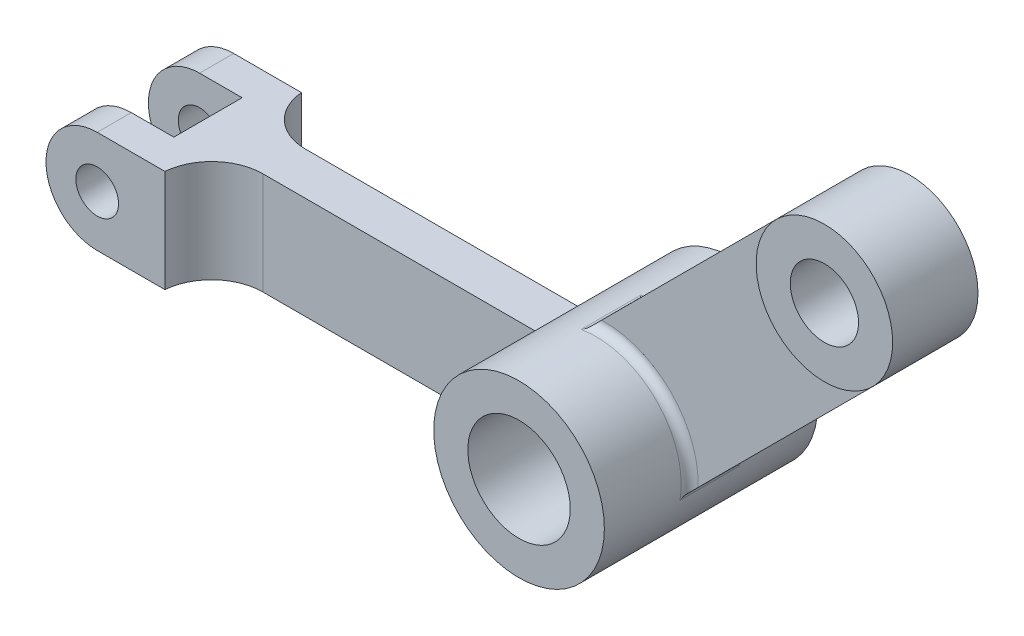
ISO-10303-21;
HEADER;
FILE_DESCRIPTION(('STEP AP214'),'2;1');
FILE_NAME('part.step','',(''),(''),'','','');
FILE_SCHEMA(('AUTOMOTIVE_DESIGN { 1 0 10303 214 1 1 1 1 }'));
ENDSEC;
DATA;
#1=APPLICATION_CONTEXT('core data for automotive mechanical design processes');
#2=APPLICATION_PROTOCOL_DEFINITION('international standard','automotive_design',2000,#1);
#3=PRODUCT_CONTEXT('',#1,'mechanical');
#4=PRODUCT('Part','Part','',(#3));
#5=PRODUCT_RELATED_PRODUCT_CATEGORY('part','',(#4));
#6=PRODUCT_DEFINITION_FORMATION('','',#4);
#7=PRODUCT_DEFINITION_CONTEXT('part definition',#1,'design');
#8=PRODUCT_DEFINITION('design','',#6,#7);
#9=PRODUCT_DEFINITION_SHAPE('','',#8);
#10=(LENGTH_UNIT() NAMED_UNIT(*) SI_UNIT(.MILLI.,.METRE.));
#11=(NAMED_UNIT(*) PLANE_ANGLE_UNIT() SI_UNIT($,.RADIAN.));
#12=(NAMED_UNIT(*) SI_UNIT($,.STERADIAN.) SOLID_ANGLE_UNIT());
#13=UNCERTAINTY_MEASURE_WITH_UNIT(LENGTH_MEASURE(1.E-05),#10,'distance_accuracy_value','');
#14=(GEOMETRIC_REPRESENTATION_CONTEXT(3) GLOBAL_UNCERTAINTY_ASSIGNED_CONTEXT((#13)) GLOBAL_UNIT_ASSIGNED_CONTEXT((#10,
#11,#12)) REPRESENTATION_CONTEXT('',''));
#15=CARTESIAN_POINT('',(0.,0.,0.));
#16=DIRECTION('',(0.,0.,1.));
#17=DIRECTION('',(1.,0.,0.));
#18=AXIS2_PLACEMENT_3D('',#15,#16,#17);
#19=CARTESIAN_POINT('',(0.,0.,25.));
#20=DIRECTION('',(0.,0.,1.));
#21=DIRECTION('',(1.,0.,0.));
#22=AXIS2_PLACEMENT_3D('',#19,#20,#21);
#23=PLANE('',#22);
#24=CARTESIAN_POINT('',(0.,0.,25.));
#25=DIRECTION('',(0.,0.,1.));
#26=DIRECTION('',(1.,0.,0.));
#27=AXIS2_PLACEMENT_3D('',#24,#25,#26);
#28=CIRCLE('',#27,10.);
#29=CARTESIAN_POINT('',(10.,0.,25.));
#30=VERTEX_POINT('',#29);
#31=EDGE_CURVE('E304',#30,#30,#28,.T.);
#32=ORIENTED_EDGE('',*,*,#31,.T.);
#33=EDGE_LOOP('',(#32));
#34=FACE_BOUND('',#33,.T.);
#35=CARTESIAN_POINT('',(0.,0.,25.));
#36=DIRECTION('',(0.,0.,1.));
#37=DIRECTION('',(1.,0.,0.));
#38=AXIS2_PLACEMENT_3D('',#35,#36,#37);
#39=CIRCLE('',#38,6.);
#40=CARTESIAN_POINT('',(6.,0.,25.));
#41=VERTEX_POINT('',#40);
#42=EDGE_CURVE('E299',#41,#41,#39,.T.);
#43=ORIENTED_EDGE('',*,*,#42,.F.);
#44=EDGE_LOOP('',(#43));
#45=FACE_BOUND('',#44,.T.);
#46=ADVANCED_FACE('F39',(#34,#45),#23,.T.);
#47=CARTESIAN_POINT('',(0.,0.,0.));
#48=DIRECTION('',(0.,0.,1.));
#49=DIRECTION('',(1.,0.,0.));
#50=AXIS2_PLACEMENT_3D('',#47,#48,#49);
#51=PLANE('',#50);
#52=CARTESIAN_POINT('',(0.,0.,0.));
#53=DIRECTION('',(0.,0.,1.));
#54=DIRECTION('',(1.,0.,0.));
#55=AXIS2_PLACEMENT_3D('',#52,#53,#54);
#56=CIRCLE('',#55,10.);
#57=CARTESIAN_POINT('',(10.,0.,0.));
#58=VERTEX_POINT('',#57);
#59=EDGE_CURVE('E305',#58,#58,#56,.T.);
#60=ORIENTED_EDGE('',*,*,#59,.F.);
#61=EDGE_LOOP('',(#60));
#62=FACE_BOUND('',#61,.T.);
#63=CARTESIAN_POINT('',(0.,0.,0.));
#64=DIRECTION('',(0.,0.,1.));
#65=DIRECTION('',(1.,0.,0.));
#66=AXIS2_PLACEMENT_3D('',#63,#64,#65);
#67=CIRCLE('',#66,6.);
#68=CARTESIAN_POINT('',(6.,0.,0.));
#69=VERTEX_POINT('',#68);
#70=EDGE_CURVE('E294',#69,#69,#67,.T.);
#71=ORIENTED_EDGE('',*,*,#70,.T.);
#72=EDGE_LOOP('',(#71));
#73=FACE_BOUND('',#72,.T.);
#74=ADVANCED_FACE('F412',(#62,#73),#51,.F.);
#75=CARTESIAN_POINT('',(0.,0.,25.));
#76=DIRECTION('',(0.,0.,-1.));
#77=DIRECTION('',(-1.,0.,0.));
#78=AXIS2_PLACEMENT_3D('',#75,#76,#77);
#79=CYLINDRICAL_SURFACE('',#78,10.);
#80=CARTESIAN_POINT('',(0.,0.,16.));
#81=DIRECTION('',(0.,0.,1.));
#82=DIRECTION('',(1.,0.,0.));
#83=AXIS2_PLACEMENT_3D('',#80,#81,#82);
#84=CIRCLE('',#83,10.);
#85=CARTESIAN_POINT('',(9.85099725970773,-1.71984097789032,16.));
#86=VERTEX_POINT('',#85);
#87=CARTESIAN_POINT('',(-1.71984097789032,9.85099725970773,16.));
#88=VERTEX_POINT('',#87);
#89=EDGE_CURVE('E339',#86,#88,#84,.T.);
#90=ORIENTED_EDGE('',*,*,#89,.T.);
#91=DIRECTION('',(0.,0.,-1.));
#92=VECTOR('',#91,1.);
#93=CARTESIAN_POINT('',(-1.71984097789032,9.85099725970773,25.));
#94=LINE('',#93,#92);
#95=CARTESIAN_POINT('',(-1.71984097789032,9.85099725970773,9.));
#96=VERTEX_POINT('',#95);
#97=EDGE_CURVE('E344',#88,#96,#94,.T.);
#98=ORIENTED_EDGE('',*,*,#97,.T.);
#99=CARTESIAN_POINT('',(0.,0.,9.));
#100=DIRECTION('',(0.,0.,1.));
#101=DIRECTION('',(1.,0.,0.));
#102=AXIS2_PLACEMENT_3D('',#99,#100,#101);
#103=CIRCLE('',#102,10.);
#104=CARTESIAN_POINT('',(9.85099725970773,-1.71984097789032,9.));
#105=VERTEX_POINT('',#104);
#106=EDGE_CURVE('E334',#96,#105,#103,.F.);
#107=ORIENTED_EDGE('',*,*,#106,.T.);
#108=DIRECTION('',(0.,0.,-1.));
#109=VECTOR('',#108,1.);
#110=CARTESIAN_POINT('',(9.85099725970773,-1.71984097789032,25.));
#111=LINE('',#110,#109);
#112=EDGE_CURVE('E340',#105,#86,#111,.F.);
#113=ORIENTED_EDGE('',*,*,#112,.T.);
#114=EDGE_LOOP('',(#90,#98,#107,#113));
#115=FACE_BOUND('',#114,.T.);
#116=DIRECTION('',(0.,0.,-1.));
#117=VECTOR('',#116,1.);
#118=CARTESIAN_POINT('',(-8.,6.,25.));
#119=LINE('',#118,#117);
#120=CARTESIAN_POINT('',(-8.,6.,15.));
#121=VERTEX_POINT('',#120);
#122=CARTESIAN_POINT('',(-8.,6.,10.));
#123=VERTEX_POINT('',#122);
#124=EDGE_CURVE('E312',#121,#123,#119,.T.);
#125=ORIENTED_EDGE('',*,*,#124,.F.);
#126=CARTESIAN_POINT('',(0.,0.,15.));
#127=DIRECTION('',(0.,0.,1.));
#128=DIRECTION('',(1.,0.,0.));
#129=AXIS2_PLACEMENT_3D('',#126,#127,#128);
#130=CIRCLE('',#129,10.);
#131=CARTESIAN_POINT('',(-8.,-6.,15.));
#132=VERTEX_POINT('',#131);
#133=EDGE_CURVE('E316',#121,#132,#130,.T.);
#134=ORIENTED_EDGE('',*,*,#133,.T.);
#135=DIRECTION('',(0.,0.,-1.));
#136=VECTOR('',#135,1.);
#137=CARTESIAN_POINT('',(-8.,-6.,25.));
#138=LINE('',#137,#136);
#139=CARTESIAN_POINT('',(-8.,-6.,10.));
#140=VERTEX_POINT('',#139);
#141=EDGE_CURVE('E317',#140,#132,#138,.F.);
#142=ORIENTED_EDGE('',*,*,#141,.F.);
#143=CARTESIAN_POINT('',(0.,0.,10.));
#144=DIRECTION('',(0.,0.,1.));
#145=DIRECTION('',(1.,0.,0.));
#146=AXIS2_PLACEMENT_3D('',#143,#144,#145);
#147=CIRCLE('',#146,10.);
#148=EDGE_CURVE('E308',#123,#140,#147,.T.);
#149=ORIENTED_EDGE('',*,*,#148,.F.);
#150=EDGE_LOOP('',(#125,#134,#142,#149));
#151=FACE_BOUND('',#150,.T.);
#152=ORIENTED_EDGE('',*,*,#31,.F.);
#153=EDGE_LOOP('',(#152));
#154=FACE_BOUND('',#153,.T.);
#155=ORIENTED_EDGE('',*,*,#59,.T.);
#156=EDGE_LOOP('',(#155));
#157=FACE_BOUND('',#156,.T.);
#158=ADVANCED_FACE('F414',(#115,#151,#154,#157),#79,.T.);
#159=CARTESIAN_POINT('',(0.,0.,25.));
#160=DIRECTION('',(0.,0.,-1.));
#161=DIRECTION('',(-1.,0.,0.));
#162=AXIS2_PLACEMENT_3D('',#159,#160,#161);
#163=CYLINDRICAL_SURFACE('',#162,6.);
#164=ORIENTED_EDGE('',*,*,#42,.T.);
#165=EDGE_LOOP('',(#164));
#166=FACE_BOUND('',#165,.T.);
#167=ORIENTED_EDGE('',*,*,#70,.F.);
#168=EDGE_LOOP('',(#167));
#169=FACE_BOUND('',#168,.T.);
#170=ADVANCED_FACE('F413',(#166,#169),#163,.F.);
#171=CARTESIAN_POINT('',(-46.,-6.,15.));
#172=DIRECTION('',(0.,1.,0.));
#173=DIRECTION('',(0.,0.,1.));
#174=AXIS2_PLACEMENT_3D('',#171,#172,#173);
#175=PLANE('',#174);
#176=DIRECTION('',(1.,0.,0.));
#177=VECTOR('',#176,1.);
#178=CARTESIAN_POINT('',(-46.,-6.,4.5));
#179=LINE('',#178,#177);
#180=CARTESIAN_POINT('',(-53.9333097995708,-6.,4.5));
#181=VERTEX_POINT('',#180);
#182=CARTESIAN_POINT('',(-46.,-6.,4.5));
#183=VERTEX_POINT('',#182);
#184=EDGE_CURVE('E267',#181,#183,#179,.T.);
#185=ORIENTED_EDGE('',*,*,#184,.T.);
#186=CARTESIAN_POINT('',(-40.0208696284493,-6.,4.));
#187=DIRECTION('',(0.,1.,0.));
#188=DIRECTION('',(0.,0.,1.));
#189=AXIS2_PLACEMENT_3D('',#186,#187,#188);
#190=CIRCLE('',#189,6.);
#191=CARTESIAN_POINT('',(-40.0208696284493,-6.,10.));
#192=VERTEX_POINT('',#191);
#193=EDGE_CURVE('E326',#183,#192,#190,.T.);
#194=ORIENTED_EDGE('',*,*,#193,.T.);
#195=DIRECTION('',(1.,0.,0.));
#196=VECTOR('',#195,1.);
#197=CARTESIAN_POINT('',(-46.,-6.,10.));
#198=LINE('',#197,#196);
#199=EDGE_CURVE('E283',#192,#140,#198,.T.);
#200=ORIENTED_EDGE('',*,*,#199,.T.);
#201=ORIENTED_EDGE('',*,*,#141,.T.);
#202=DIRECTION('',(1.,0.,0.));
#203=VECTOR('',#202,1.);
#204=CARTESIAN_POINT('',(-46.,-6.,15.));
#205=LINE('',#204,#203);
#206=CARTESIAN_POINT('',(-40.0208696284493,-6.,15.));
#207=VERTEX_POINT('',#206);
#208=EDGE_CURVE('E287',#207,#132,#205,.T.);
#209=ORIENTED_EDGE('',*,*,#208,.F.);
#210=CARTESIAN_POINT('',(-40.0208696284493,-6.,21.));
#211=DIRECTION('',(0.,1.,0.));
#212=DIRECTION('',(0.,0.,1.));
#213=AXIS2_PLACEMENT_3D('',#210,#211,#212);
#214=CIRCLE('',#213,6.);
#215=CARTESIAN_POINT('',(-46.,-6.,20.5));
#216=VERTEX_POINT('',#215);
#217=EDGE_CURVE('E333',#207,#216,#214,.T.);
#218=ORIENTED_EDGE('',*,*,#217,.T.);
#219=DIRECTION('',(1.,0.,0.));
#220=VECTOR('',#219,1.);
#221=CARTESIAN_POINT('',(-46.,-6.,20.5));
#222=LINE('',#221,#220);
#223=CARTESIAN_POINT('',(-53.9333097995708,-6.,20.5));
#224=VERTEX_POINT('',#223);
#225=EDGE_CURVE('E260',#224,#216,#222,.T.);
#226=ORIENTED_EDGE('',*,*,#225,.F.);
#227=DIRECTION('',(0.,0.,-1.));
#228=VECTOR('',#227,1.);
#229=CARTESIAN_POINT('',(-53.9333097995708,-6.,20.5));
#230=LINE('',#229,#228);
#231=CARTESIAN_POINT('',(-53.9333097995708,-6.,16.5));
#232=VERTEX_POINT('',#231);
#233=EDGE_CURVE('E284',#224,#232,#230,.T.);
#234=ORIENTED_EDGE('',*,*,#233,.T.);
#235=DIRECTION('',(1.,0.,0.));
#236=VECTOR('',#235,1.);
#237=CARTESIAN_POINT('',(-46.,-6.,16.5));
#238=LINE('',#237,#236);
#239=CARTESIAN_POINT('',(-48.9536388352292,-6.,16.5));
#240=VERTEX_POINT('',#239);
#241=EDGE_CURVE('E235',#232,#240,#238,.T.);
#242=ORIENTED_EDGE('',*,*,#241,.T.);
#243=DIRECTION('',(0.,0.,-1.));
#244=VECTOR('',#243,1.);
#245=CARTESIAN_POINT('',(-48.9536388352292,-6.,20.5));
#246=LINE('',#245,#244);
#247=CARTESIAN_POINT('',(-48.9536388352292,-6.,8.5));
#248=VERTEX_POINT('',#247);
#249=EDGE_CURVE('E244',#240,#248,#246,.T.);
#250=ORIENTED_EDGE('',*,*,#249,.T.);
#251=DIRECTION('',(-1.,0.,0.));
#252=VECTOR('',#251,1.);
#253=CARTESIAN_POINT('',(-46.,-6.,8.5));
#254=LINE('',#253,#252);
#255=CARTESIAN_POINT('',(-53.9333097995708,-6.,8.5));
#256=VERTEX_POINT('',#255);
#257=EDGE_CURVE('E237',#248,#256,#254,.T.);
#258=ORIENTED_EDGE('',*,*,#257,.T.);
#259=EDGE_CURVE('E277',#256,#181,#230,.T.);
#260=ORIENTED_EDGE('',*,*,#259,.T.);
#261=EDGE_LOOP('',(#185,#194,#200,#201,#209,#218,#226,#234,#242,#250,#258,#260));
#262=FACE_BOUND('',#261,.T.);
#263=ADVANCED_FACE('F424',(#262),#175,.F.);
#264=CARTESIAN_POINT('',(-46.,6.,15.));
#265=DIRECTION('',(0.,-1.,0.));
#266=DIRECTION('',(0.,0.,-1.));
#267=AXIS2_PLACEMENT_3D('',#264,#265,#266);
#268=PLANE('',#267);
#269=DIRECTION('',(-1.,0.,0.));
#270=VECTOR('',#269,1.);
#271=CARTESIAN_POINT('',(-46.,6.,15.));
#272=LINE('',#271,#270);
#273=CARTESIAN_POINT('',(-40.0208696284493,6.,15.));
#274=VERTEX_POINT('',#273);
#275=EDGE_CURVE('E293',#121,#274,#272,.T.);
#276=ORIENTED_EDGE('',*,*,#275,.F.);
#277=ORIENTED_EDGE('',*,*,#124,.T.);
#278=DIRECTION('',(-1.,0.,0.));
#279=VECTOR('',#278,1.);
#280=CARTESIAN_POINT('',(-46.,6.,10.));
#281=LINE('',#280,#279);
#282=CARTESIAN_POINT('',(-40.0208696284493,6.,10.));
#283=VERTEX_POINT('',#282);
#284=EDGE_CURVE('E292',#123,#283,#281,.T.);
#285=ORIENTED_EDGE('',*,*,#284,.T.);
#286=CARTESIAN_POINT('',(-40.0208696284493,6.,4.));
#287=DIRECTION('',(0.,-1.,0.));
#288=DIRECTION('',(0.,0.,-1.));
#289=AXIS2_PLACEMENT_3D('',#286,#287,#288);
#290=CIRCLE('',#289,6.);
#291=CARTESIAN_POINT('',(-46.,6.,4.5));
#292=VERTEX_POINT('',#291);
#293=EDGE_CURVE('E328',#283,#292,#290,.T.);
#294=ORIENTED_EDGE('',*,*,#293,.T.);
#295=DIRECTION('',(-1.,0.,0.));
#296=VECTOR('',#295,1.);
#297=CARTESIAN_POINT('',(-53.9333097995708,6.,4.5));
#298=LINE('',#297,#296);
#299=CARTESIAN_POINT('',(-53.9333097995708,6.,4.5));
#300=VERTEX_POINT('',#299);
#301=EDGE_CURVE('E258',#292,#300,#298,.T.);
#302=ORIENTED_EDGE('',*,*,#301,.T.);
#303=DIRECTION('',(0.,0.,-1.));
#304=VECTOR('',#303,1.);
#305=CARTESIAN_POINT('',(-53.9333097995708,6.,20.5));
#306=LINE('',#305,#304);
#307=CARTESIAN_POINT('',(-53.9333097995708,6.,8.5));
#308=VERTEX_POINT('',#307);
#309=EDGE_CURVE('E268',#308,#300,#306,.T.);
#310=ORIENTED_EDGE('',*,*,#309,.F.);
#311=DIRECTION('',(-1.,0.,0.));
#312=VECTOR('',#311,1.);
#313=CARTESIAN_POINT('',(-63.6938952559095,6.,8.5));
#314=LINE('',#313,#312);
#315=CARTESIAN_POINT('',(-48.9536388352292,6.,8.5));
#316=VERTEX_POINT('',#315);
#317=EDGE_CURVE('E191',#316,#308,#314,.T.);
#318=ORIENTED_EDGE('',*,*,#317,.F.);
#319=DIRECTION('',(0.,0.,-1.));
#320=VECTOR('',#319,1.);
#321=CARTESIAN_POINT('',(-48.9536388352292,6.,8.5));
#322=LINE('',#321,#320);
#323=CARTESIAN_POINT('',(-48.9536388352292,6.,16.5));
#324=VERTEX_POINT('',#323);
#325=EDGE_CURVE('E222',#324,#316,#322,.T.);
#326=ORIENTED_EDGE('',*,*,#325,.F.);
#327=DIRECTION('',(1.,0.,0.));
#328=VECTOR('',#327,1.);
#329=CARTESIAN_POINT('',(-48.9536388352292,6.,16.5));
#330=LINE('',#329,#328);
#331=CARTESIAN_POINT('',(-53.9333097995708,6.,16.5));
#332=VERTEX_POINT('',#331);
#333=EDGE_CURVE('E223',#332,#324,#330,.T.);
#334=ORIENTED_EDGE('',*,*,#333,.F.);
#335=CARTESIAN_POINT('',(-53.9333097995708,6.,20.5));
#336=VERTEX_POINT('',#335);
#337=EDGE_CURVE('E276',#336,#332,#306,.T.);
#338=ORIENTED_EDGE('',*,*,#337,.F.);
#339=DIRECTION('',(-1.,0.,0.));
#340=VECTOR('',#339,1.);
#341=CARTESIAN_POINT('',(-53.9333097995708,6.,20.5));
#342=LINE('',#341,#340);
#343=CARTESIAN_POINT('',(-46.,6.,20.5));
#344=VERTEX_POINT('',#343);
#345=EDGE_CURVE('E263',#344,#336,#342,.T.);
#346=ORIENTED_EDGE('',*,*,#345,.F.);
#347=CARTESIAN_POINT('',(-40.0208696284493,6.,21.));
#348=DIRECTION('',(0.,-1.,0.));
#349=DIRECTION('',(0.,0.,-1.));
#350=AXIS2_PLACEMENT_3D('',#347,#348,#349);
#351=CIRCLE('',#350,6.);
#352=EDGE_CURVE('E331',#344,#274,#351,.T.);
#353=ORIENTED_EDGE('',*,*,#352,.T.);
#354=EDGE_LOOP('',(#276,#277,#285,#294,#302,#310,#318,#326,#334,#338,#346,#353));
#355=FACE_BOUND('',#354,.T.);
#356=ADVANCED_FACE('F429',(#355),#268,.F.);
#357=CARTESIAN_POINT('',(0.,0.,15.));
#358=DIRECTION('',(0.,0.,1.));
#359=DIRECTION('',(1.,0.,0.));
#360=AXIS2_PLACEMENT_3D('',#357,#358,#359);
#361=PLANE('',#360);
#362=ORIENTED_EDGE('',*,*,#275,.T.);
#363=DIRECTION('',(0.,-1.,0.));
#364=VECTOR('',#363,1.);
#365=CARTESIAN_POINT('',(-40.0208696284493,-6.,15.));
#366=LINE('',#365,#364);
#367=EDGE_CURVE('E323',#274,#207,#366,.T.);
#368=ORIENTED_EDGE('',*,*,#367,.T.);
#369=ORIENTED_EDGE('',*,*,#208,.T.);
#370=ORIENTED_EDGE('',*,*,#133,.F.);
#371=EDGE_LOOP('',(#362,#368,#369,#370));
#372=FACE_BOUND('',#371,.T.);
#373=ADVANCED_FACE('F433',(#372),#361,.T.);
#374=CARTESIAN_POINT('',(0.,0.,10.));
#375=DIRECTION('',(0.,0.,1.));
#376=DIRECTION('',(1.,0.,0.));
#377=AXIS2_PLACEMENT_3D('',#374,#375,#376);
#378=PLANE('',#377);
#379=ORIENTED_EDGE('',*,*,#199,.F.);
#380=DIRECTION('',(0.,1.,0.));
#381=VECTOR('',#380,1.);
#382=CARTESIAN_POINT('',(-40.0208696284493,0.,10.));
#383=LINE('',#382,#381);
#384=EDGE_CURVE('E321',#192,#283,#383,.T.);
#385=ORIENTED_EDGE('',*,*,#384,.T.);
#386=ORIENTED_EDGE('',*,*,#284,.F.);
#387=ORIENTED_EDGE('',*,*,#148,.T.);
#388=EDGE_LOOP('',(#379,#385,#386,#387));
#389=FACE_BOUND('',#388,.T.);
#390=ADVANCED_FACE('F434',(#389),#378,.F.);
#391=CARTESIAN_POINT('',(-53.9333097995708,0.,20.5));
#392=DIRECTION('',(0.,0.,-1.));
#393=DIRECTION('',(-1.,0.,0.));
#394=AXIS2_PLACEMENT_3D('',#391,#392,#393);
#395=CYLINDRICAL_SURFACE('',#394,6.);
#396=ORIENTED_EDGE('',*,*,#259,.F.);
#397=CARTESIAN_POINT('',(-53.9333097995708,0.,8.5));
#398=DIRECTION('',(0.,0.,-1.));
#399=DIRECTION('',(-1.,0.,0.));
#400=AXIS2_PLACEMENT_3D('',#397,#398,#399);
#401=CIRCLE('',#400,6.);
#402=EDGE_CURVE('E245',#256,#308,#401,.T.);
#403=ORIENTED_EDGE('',*,*,#402,.T.);
#404=ORIENTED_EDGE('',*,*,#309,.T.);
#405=CARTESIAN_POINT('',(-53.9333097995708,0.,4.5));
#406=DIRECTION('',(0.,0.,1.));
#407=DIRECTION('',(1.,0.,0.));
#408=AXIS2_PLACEMENT_3D('',#405,#406,#407);
#409=CIRCLE('',#408,6.);
#410=EDGE_CURVE('E255',#300,#181,#409,.T.);
#411=ORIENTED_EDGE('',*,*,#410,.T.);
#412=EDGE_LOOP('',(#396,#403,#404,#411));
#413=FACE_BOUND('',#412,.T.);
#414=ADVANCED_FACE('F438',(#413),#395,.T.);
#415=CARTESIAN_POINT('',(-53.9333097995708,0.,20.5));
#416=DIRECTION('',(0.,0.,-1.));
#417=DIRECTION('',(-1.,0.,0.));
#418=AXIS2_PLACEMENT_3D('',#415,#416,#417);
#419=CYLINDRICAL_SURFACE('',#418,2.5);
#420=CARTESIAN_POINT('',(-53.9333097995708,0.,8.5));
#421=DIRECTION('',(0.,0.,-1.));
#422=DIRECTION('',(-1.,0.,0.));
#423=AXIS2_PLACEMENT_3D('',#420,#421,#422);
#424=CIRCLE('',#423,2.5);
#425=CARTESIAN_POINT('',(-56.4333097995708,0.,8.5));
#426=VERTEX_POINT('',#425);
#427=EDGE_CURVE('E238',#426,#426,#424,.T.);
#428=ORIENTED_EDGE('',*,*,#427,.F.);
#429=EDGE_LOOP('',(#428));
#430=FACE_BOUND('',#429,.T.);
#431=CARTESIAN_POINT('',(-53.9333097995708,0.,4.5));
#432=DIRECTION('',(0.,0.,1.));
#433=DIRECTION('',(1.,0.,0.));
#434=AXIS2_PLACEMENT_3D('',#431,#432,#433);
#435=CIRCLE('',#434,2.5);
#436=CARTESIAN_POINT('',(-51.4333097995708,0.,4.5));
#437=VERTEX_POINT('',#436);
#438=EDGE_CURVE('E247',#437,#437,#435,.T.);
#439=ORIENTED_EDGE('',*,*,#438,.F.);
#440=EDGE_LOOP('',(#439));
#441=FACE_BOUND('',#440,.T.);
#442=ADVANCED_FACE('F452',(#430,#441),#419,.F.);
#443=CARTESIAN_POINT('',(-53.9333097995708,0.,20.5));
#444=DIRECTION('',(0.,0.,1.));
#445=DIRECTION('',(1.,0.,0.));
#446=AXIS2_PLACEMENT_3D('',#443,#444,#445);
#447=PLANE('',#446);
#448=CARTESIAN_POINT('',(-53.9333097995708,0.,20.5));
#449=DIRECTION('',(0.,0.,1.));
#450=DIRECTION('',(1.,0.,0.));
#451=AXIS2_PLACEMENT_3D('',#448,#449,#450);
#452=CIRCLE('',#451,6.);
#453=EDGE_CURVE('E253',#336,#224,#452,.T.);
#454=ORIENTED_EDGE('',*,*,#453,.T.);
#455=ORIENTED_EDGE('',*,*,#225,.T.);
#456=DIRECTION('',(0.,1.,0.));
#457=VECTOR('',#456,1.);
#458=CARTESIAN_POINT('',(-46.,6.,20.5));
#459=LINE('',#458,#457);
#460=EDGE_CURVE('E261',#216,#344,#459,.T.);
#461=ORIENTED_EDGE('',*,*,#460,.T.);
#462=ORIENTED_EDGE('',*,*,#345,.T.);
#463=EDGE_LOOP('',(#454,#455,#461,#462));
#464=FACE_BOUND('',#463,.T.);
#465=CARTESIAN_POINT('',(-53.9333097995708,0.,20.5));
#466=DIRECTION('',(0.,0.,1.));
#467=DIRECTION('',(1.,0.,0.));
#468=AXIS2_PLACEMENT_3D('',#465,#466,#467);
#469=CIRCLE('',#468,2.5);
#470=CARTESIAN_POINT('',(-51.4333097995708,0.,20.5));
#471=VERTEX_POINT('',#470);
#472=EDGE_CURVE('E248',#471,#471,#469,.T.);
#473=ORIENTED_EDGE('',*,*,#472,.F.);
#474=EDGE_LOOP('',(#473));
#475=FACE_BOUND('',#474,.T.);
#476=ADVANCED_FACE('F454',(#464,#475),#447,.T.);
#477=CARTESIAN_POINT('',(-53.9333097995708,0.,4.5));
#478=DIRECTION('',(0.,0.,1.));
#479=DIRECTION('',(1.,0.,0.));
#480=AXIS2_PLACEMENT_3D('',#477,#478,#479);
#481=PLANE('',#480);
#482=ORIENTED_EDGE('',*,*,#410,.F.);
#483=ORIENTED_EDGE('',*,*,#301,.F.);
#484=DIRECTION('',(0.,1.,0.));
#485=VECTOR('',#484,1.);
#486=CARTESIAN_POINT('',(-46.,6.,4.5));
#487=LINE('',#486,#485);
#488=EDGE_CURVE('E275',#183,#292,#487,.T.);
#489=ORIENTED_EDGE('',*,*,#488,.F.);
#490=ORIENTED_EDGE('',*,*,#184,.F.);
#491=EDGE_LOOP('',(#482,#483,#489,#490));
#492=FACE_BOUND('',#491,.T.);
#493=ORIENTED_EDGE('',*,*,#438,.T.);
#494=EDGE_LOOP('',(#493));
#495=FACE_BOUND('',#494,.T.);
#496=ADVANCED_FACE('F450',(#492,#495),#481,.F.);
#497=ORIENTED_EDGE('',*,*,#337,.T.);
#498=CARTESIAN_POINT('',(-53.9333097995708,0.,16.5));
#499=DIRECTION('',(0.,0.,1.));
#500=DIRECTION('',(1.,0.,0.));
#501=AXIS2_PLACEMENT_3D('',#498,#499,#500);
#502=CIRCLE('',#501,6.);
#503=EDGE_CURVE('E232',#332,#232,#502,.T.);
#504=ORIENTED_EDGE('',*,*,#503,.T.);
#505=ORIENTED_EDGE('',*,*,#233,.F.);
#506=ORIENTED_EDGE('',*,*,#453,.F.);
#507=EDGE_LOOP('',(#497,#504,#505,#506));
#508=FACE_BOUND('',#507,.T.);
#509=ADVANCED_FACE('F442',(#508),#395,.T.);
#510=CARTESIAN_POINT('',(-53.9333097995708,0.,16.5));
#511=DIRECTION('',(0.,0.,1.));
#512=DIRECTION('',(1.,0.,0.));
#513=AXIS2_PLACEMENT_3D('',#510,#511,#512);
#514=CIRCLE('',#513,2.5);
#515=CARTESIAN_POINT('',(-51.4333097995708,0.,16.5));
#516=VERTEX_POINT('',#515);
#517=EDGE_CURVE('E229',#516,#516,#514,.T.);
#518=ORIENTED_EDGE('',*,*,#517,.F.);
#519=EDGE_LOOP('',(#518));
#520=FACE_BOUND('',#519,.T.);
#521=ORIENTED_EDGE('',*,*,#472,.T.);
#522=EDGE_LOOP('',(#521));
#523=FACE_BOUND('',#522,.T.);
#524=ADVANCED_FACE('F447',(#520,#523),#419,.F.);
#525=CARTESIAN_POINT('',(-48.9536388352292,-10.,8.5));
#526=DIRECTION('',(1.,0.,0.));
#527=DIRECTION('',(0.,0.,-1.));
#528=AXIS2_PLACEMENT_3D('',#525,#526,#527);
#529=PLANE('',#528);
#530=DIRECTION('',(0.,1.,0.));
#531=VECTOR('',#530,1.);
#532=CARTESIAN_POINT('',(-48.9536388352292,-10.,16.5));
#533=LINE('',#532,#531);
#534=EDGE_CURVE('E227',#240,#324,#533,.T.);
#535=ORIENTED_EDGE('',*,*,#534,.T.);
#536=ORIENTED_EDGE('',*,*,#325,.T.);
#537=DIRECTION('',(0.,1.,0.));
#538=VECTOR('',#537,1.);
#539=CARTESIAN_POINT('',(-48.9536388352292,-10.,8.5));
#540=LINE('',#539,#538);
#541=EDGE_CURVE('E226',#248,#316,#540,.T.);
#542=ORIENTED_EDGE('',*,*,#541,.F.);
#543=ORIENTED_EDGE('',*,*,#249,.F.);
#544=EDGE_LOOP('',(#535,#536,#542,#543));
#545=FACE_BOUND('',#544,.T.);
#546=ADVANCED_FACE('F458',(#545),#529,.F.);
#547=CARTESIAN_POINT('',(-63.6938952559095,-10.,8.5));
#548=DIRECTION('',(0.,0.,-1.));
#549=DIRECTION('',(-1.,0.,0.));
#550=AXIS2_PLACEMENT_3D('',#547,#548,#549);
#551=PLANE('',#550);
#552=ORIENTED_EDGE('',*,*,#427,.T.);
#553=EDGE_LOOP('',(#552));
#554=FACE_BOUND('',#553,.T.);
#555=ORIENTED_EDGE('',*,*,#257,.F.);
#556=ORIENTED_EDGE('',*,*,#541,.T.);
#557=ORIENTED_EDGE('',*,*,#317,.T.);
#558=ORIENTED_EDGE('',*,*,#402,.F.);
#559=EDGE_LOOP('',(#555,#556,#557,#558));
#560=FACE_BOUND('',#559,.T.);
#561=ADVANCED_FACE('F463',(#554,#560),#551,.F.);
#562=CARTESIAN_POINT('',(-48.9536388352292,-10.,16.5));
#563=DIRECTION('',(0.,0.,1.));
#564=DIRECTION('',(1.,0.,0.));
#565=AXIS2_PLACEMENT_3D('',#562,#563,#564);
#566=PLANE('',#565);
#567=ORIENTED_EDGE('',*,*,#517,.T.);
#568=EDGE_LOOP('',(#567));
#569=FACE_BOUND('',#568,.T.);
#570=ORIENTED_EDGE('',*,*,#333,.T.);
#571=ORIENTED_EDGE('',*,*,#534,.F.);
#572=ORIENTED_EDGE('',*,*,#241,.F.);
#573=ORIENTED_EDGE('',*,*,#503,.F.);
#574=EDGE_LOOP('',(#570,#571,#572,#573));
#575=FACE_BOUND('',#574,.T.);
#576=ADVANCED_FACE('F462',(#569,#575),#566,.F.);
#577=CARTESIAN_POINT('',(-1.4142135623731,9.89949493661167,15.));
#578=DIRECTION('',(0.707106781186547,-0.707106781186548,0.));
#579=DIRECTION('',(0.707106781186548,0.707106781186547,0.));
#580=AXIS2_PLACEMENT_3D('',#577,#578,#579);
#581=PLANE('',#580);
#582=DIRECTION('',(-0.707106781186548,-0.707106781186547,0.));
#583=VECTOR('',#582,1.);
#584=CARTESIAN_POINT('',(-1.4142135623731,9.89949493661167,10.));
#585=LINE('',#584,#583);
#586=CARTESIAN_POINT('',(22.6274169979695,33.9411254969543,10.));
#587=VERTEX_POINT('',#586);
#588=CARTESIAN_POINT('',(-0.318315123476729,10.995393375508,10.));
#589=VERTEX_POINT('',#588);
#590=EDGE_CURVE('E183',#587,#589,#585,.T.);
#591=ORIENTED_EDGE('',*,*,#590,.T.);
#592=CARTESIAN_POINT('',(-0.318315123476729,10.995393375508,10.));
#593=CARTESIAN_POINT('',(-0.362148546825368,10.9515599521594,9.9999823517167));
#594=CARTESIAN_POINT('',(-0.405978283879837,10.9077302151049,9.99728398431099));
#595=CARTESIAN_POINT('',(-0.493328584937231,10.8203799140475,9.98661260035009));
#596=CARTESIAN_POINT('',(-0.536849057465292,10.7768594415195,9.97863808388791));
#597=CARTESIAN_POINT('',(-0.621938071444188,10.6917704275406,9.95782314668862));
#598=CARTESIAN_POINT('',(-0.663525694382294,10.6501828046025,9.9451383060557));
#599=CARTESIAN_POINT('',(-0.74580163336438,10.5679068656204,9.91484655018754));
#600=CARTESIAN_POINT('',(-0.78648997133472,10.52721852765,9.89723975510252));
#601=CARTESIAN_POINT('',(-0.858434273365647,10.4552742256191,9.86105904173088));
#602=CARTESIAN_POINT('',(-0.889923844930278,10.4237846540545,9.84341207935038));
#603=CARTESIAN_POINT('',(-0.951837031903636,10.3618714670811,9.80477554674164));
#604=CARTESIAN_POINT('',(-0.982261443174357,10.3314470558104,9.78378854007573));
#605=CARTESIAN_POINT('',(-1.04250589005114,10.2712026089336,9.73770722777967));
#606=CARTESIAN_POINT('',(-1.07229252061271,10.2414159783721,9.71252439929404));
#607=CARTESIAN_POINT('',(-1.13003032316563,10.1836781758191,9.65808072325631));
#608=CARTESIAN_POINT('',(-1.15797710439665,10.1557313945881,9.62881060611017));
#609=CARTESIAN_POINT('',(-1.18471829449286,10.1289902044919,9.59737642913233));
#610=B_SPLINE_CURVE_WITH_KNOTS('',3,(#592,#593,#594,#595,#596,#597,#598,#599,#600,#601,#602,
#603,#604,#605,#606,#607,#608,#609),.UNSPECIFIED.,.F.,.F.,(4,2,2,2,2,2,2,2,4),(0.,
0.1859060498299,0.371864971869382,0.55216077313547,0.732452173570472,0.876031905451659,
1.01950196331913,1.16650996428862,1.3138569506875),.UNSPECIFIED.);
#611=CARTESIAN_POINT('',(-1.18471829449281,10.128990204492,9.5973764291321));
#612=VERTEX_POINT('',#611);
#613=EDGE_CURVE('E11',#589,#612,#610,.T.);
#614=ORIENTED_EDGE('',*,*,#613,.T.);
#615=DIRECTION('',(0.,0.,1.));
#616=VECTOR('',#615,1.);
#617=CARTESIAN_POINT('',(-1.18471829449281,10.128990204492,15.));
#618=LINE('',#617,#616);
#619=CARTESIAN_POINT('',(-1.18471829449281,10.128990204492,15.4026235708679));
#620=VERTEX_POINT('',#619);
#621=EDGE_CURVE('E343',#612,#620,#618,.T.);
#622=ORIENTED_EDGE('',*,*,#621,.T.);
#623=CARTESIAN_POINT('',(-1.18471829449281,10.128990204492,15.4026235708679));
#624=CARTESIAN_POINT('',(-1.16158549816465,10.1521230008201,15.3754162721457));
#625=CARTESIAN_POINT('',(-1.13753785541226,10.1761706435725,15.3498335739045));
#626=CARTESIAN_POINT('',(-1.0879994436789,10.2257090553059,15.3017613562249));
#627=CARTESIAN_POINT('',(-1.06251124479582,10.2511972541889,15.2792665591668));
#628=CARTESIAN_POINT('',(-1.01043271040665,10.3032757885781,15.2371511383471));
#629=CARTESIAN_POINT('',(-0.983843986250528,10.3298645127342,15.2175264907706));
#630=CARTESIAN_POINT('',(-0.929747085352385,10.3839614136324,15.1809536811205));
#631=CARTESIAN_POINT('',(-0.902238348339115,10.4114701506457,15.1640071873257));
#632=CARTESIAN_POINT('',(-0.835390995015036,10.4783175039697,15.1264463481603));
#633=CARTESIAN_POINT('',(-0.795704410293197,10.5180040886916,15.1070593500486));
#634=CARTESIAN_POINT('',(-0.715306082457799,10.598402416527,15.0731160705763));
#635=CARTESIAN_POINT('',(-0.67459354313478,10.63911495585,15.0585636736903));
#636=CARTESIAN_POINT('',(-0.551416010319706,10.7622924886651,15.0220496103511));
#637=CARTESIAN_POINT('',(-0.467797714317564,10.8459107846672,15.0071690002344));
#638=CARTESIAN_POINT('',(-0.373098398801382,10.9406101001834,15.0013515146159));
#639=CARTESIAN_POINT('',(-0.362135303132082,10.9515731958527,15.0008449890677));
#640=CARTESIAN_POINT('',(-0.340220881358781,10.973487617626,15.0001694452766));
#641=CARTESIAN_POINT('',(-0.329269563271265,10.9844389357135,14.999999906319));
#642=CARTESIAN_POINT('',(-0.31831512347673,10.995393375508,15.));
#643=B_SPLINE_CURVE_WITH_KNOTS('',3,(#623,#624,#625,#626,#627,#628,#629,#630,#631,#632,#633,
#634,#635,#636,#637,#638,#639,#640,#641,#642),.UNSPECIFIED.,.F.,.F.,(4,2,2,2,2,2,2,2,2,4),(0.,
0.127534814868873,0.254848867728498,0.381982685169961,0.509195387441639,0.68707447370762,
0.865096137416619,1.22062916296543,1.26716716093884,1.31363319189916),.UNSPECIFIED.);
#644=CARTESIAN_POINT('',(-0.31831512347673,10.995393375508,15.));
#645=VERTEX_POINT('',#644);
#646=EDGE_CURVE('E357',#620,#645,#643,.T.);
#647=ORIENTED_EDGE('',*,*,#646,.T.);
#648=DIRECTION('',(-0.707106781186548,-0.707106781186547,0.));
#649=VECTOR('',#648,1.);
#650=CARTESIAN_POINT('',(-1.4142135623731,9.89949493661167,15.));
#651=LINE('',#650,#649);
#652=CARTESIAN_POINT('',(22.6274169979695,33.9411254969543,15.));
#653=VERTEX_POINT('',#652);
#654=EDGE_CURVE('E190',#653,#645,#651,.T.);
#655=ORIENTED_EDGE('',*,*,#654,.F.);
#656=DIRECTION('',(0.,0.,-1.));
#657=VECTOR('',#656,1.);
#658=CARTESIAN_POINT('',(22.6274169979695,33.9411254969543,15.));
#659=LINE('',#658,#657);
#660=EDGE_CURVE('E181',#653,#587,#659,.T.);
#661=ORIENTED_EDGE('',*,*,#660,.T.);
#662=EDGE_LOOP('',(#591,#614,#622,#647,#655,#661));
#663=FACE_BOUND('',#662,.T.);
#664=ADVANCED_FACE('F182',(#663),#581,.F.);
#665=CARTESIAN_POINT('',(9.89949493661167,-1.4142135623731,15.));
#666=DIRECTION('',(-0.707106781186548,0.707106781186547,0.));
#667=DIRECTION('',(-0.707106781186547,-0.707106781186548,0.));
#668=AXIS2_PLACEMENT_3D('',#665,#666,#667);
#669=PLANE('',#668);
#670=CARTESIAN_POINT('',(10.995393375508,-0.318315123476731,15.));
#671=CARTESIAN_POINT('',(10.9515599521594,-0.362148546825368,15.0000176482833));
#672=CARTESIAN_POINT('',(10.9077302151049,-0.405978283879837,15.002716015689));
#673=CARTESIAN_POINT('',(10.8203799140475,-0.493328584937232,15.0133873996499));
#674=CARTESIAN_POINT('',(10.7768594415195,-0.536849057465293,15.0213619161121));
#675=CARTESIAN_POINT('',(10.6917704275406,-0.62193807144419,15.0421768533114));
#676=CARTESIAN_POINT('',(10.6501828046025,-0.663525694382295,15.0548616939443));
#677=CARTESIAN_POINT('',(10.5679068656204,-0.745801633364381,15.0851534498125));
#678=CARTESIAN_POINT('',(10.52721852765,-0.786489971334721,15.1027602448975));
#679=CARTESIAN_POINT('',(10.4552742256191,-0.858434273365648,15.1389409582691));
#680=CARTESIAN_POINT('',(10.4237846540545,-0.889923844930279,15.1565879206496));
#681=CARTESIAN_POINT('',(10.3618714670811,-0.951837031903637,15.1952244532584));
#682=CARTESIAN_POINT('',(10.3314470558104,-0.982261443174357,15.2162114599243));
#683=CARTESIAN_POINT('',(10.2712026089336,-1.04250589005114,15.2622927722203));
#684=CARTESIAN_POINT('',(10.2414159783721,-1.07229252061271,15.287475600706));
#685=CARTESIAN_POINT('',(10.1836781758191,-1.13003032316563,15.3419192767437));
#686=CARTESIAN_POINT('',(10.1557313945881,-1.15797710439665,15.3711893938898));
#687=CARTESIAN_POINT('',(10.1289902044919,-1.18471829449286,15.4026235708677));
#688=B_SPLINE_CURVE_WITH_KNOTS('',3,(#670,#671,#672,#673,#674,#675,#676,#677,#678,#679,#680,
#681,#682,#683,#684,#685,#686,#687),.UNSPECIFIED.,.F.,.F.,(4,2,2,2,2,2,2,2,4),(0.,
0.185906049829901,0.371864971869382,0.552160773135471,0.732452173570474,0.876031905451658,
1.01950196331913,1.16650996428862,1.3138569506875),.UNSPECIFIED.);
#689=CARTESIAN_POINT('',(10.995393375508,-0.31831512347673,15.));
#690=VERTEX_POINT('',#689);
#691=CARTESIAN_POINT('',(10.128990204492,-1.18471829449281,15.4026235708679));
#692=VERTEX_POINT('',#691);
#693=EDGE_CURVE('E347',#690,#692,#688,.T.);
#694=ORIENTED_EDGE('',*,*,#693,.T.);
#695=DIRECTION('',(0.,0.,1.));
#696=VECTOR('',#695,1.);
#697=CARTESIAN_POINT('',(10.128990204492,-1.18471829449281,10.));
#698=LINE('',#697,#696);
#699=CARTESIAN_POINT('',(10.128990204492,-1.18471829449281,9.5973764291321));
#700=VERTEX_POINT('',#699);
#701=EDGE_CURVE('E64',#692,#700,#698,.F.);
#702=ORIENTED_EDGE('',*,*,#701,.T.);
#703=CARTESIAN_POINT('',(10.128990204492,-1.18471829449281,9.5973764291321));
#704=CARTESIAN_POINT('',(10.1521230008201,-1.16158549816465,9.6245837278543));
#705=CARTESIAN_POINT('',(10.1761706435725,-1.13753785541226,9.65016642609549));
#706=CARTESIAN_POINT('',(10.2257090553059,-1.0879994436789,9.69823864377506));
#707=CARTESIAN_POINT('',(10.2511972541889,-1.06251124479582,9.72073344083315));
#708=CARTESIAN_POINT('',(10.3032757885781,-1.01043271040665,9.76284886165291));
#709=CARTESIAN_POINT('',(10.3298645127342,-0.983843986250528,9.78247350922936));
#710=CARTESIAN_POINT('',(10.3839614136324,-0.929747085352385,9.81904631887953));
#711=CARTESIAN_POINT('',(10.4114701506457,-0.902238348339115,9.83599281267429));
#712=CARTESIAN_POINT('',(10.4783175039697,-0.835390995015036,9.87355365183972));
#713=CARTESIAN_POINT('',(10.5180040886916,-0.795704410293197,9.89294064995138));
#714=CARTESIAN_POINT('',(10.598402416527,-0.715306082457799,9.92688392942374));
#715=CARTESIAN_POINT('',(10.63911495585,-0.67459354313478,9.94143632630967));
#716=CARTESIAN_POINT('',(10.7622924886651,-0.551416010319706,9.97795038964889));
#717=CARTESIAN_POINT('',(10.8459107846672,-0.467797714317564,9.99283099976559));
#718=CARTESIAN_POINT('',(10.9406101001834,-0.373098398801383,9.99864848538409));
#719=CARTESIAN_POINT('',(10.9515731958527,-0.362135303132082,9.99915501093226));
#720=CARTESIAN_POINT('',(10.973487617626,-0.340220881358781,9.99983055472336));
#721=CARTESIAN_POINT('',(10.9844389357135,-0.329269563271265,10.000000093681));
#722=CARTESIAN_POINT('',(10.995393375508,-0.31831512347673,10.));
#723=B_SPLINE_CURVE_WITH_KNOTS('',3,(#703,#704,#705,#706,#707,#708,#709,#710,#711,#712,#713,
#714,#715,#716,#717,#718,#719,#720,#721,#722),.UNSPECIFIED.,.F.,.F.,(4,2,2,2,2,2,2,2,2,4),(0.,
0.127534814868873,0.254848867728498,0.381982685169961,0.509195387441639,0.687074473707621,
0.865096137416618,1.22062916296543,1.26716716093884,1.31363319189916),.UNSPECIFIED.);
#724=CARTESIAN_POINT('',(10.995393375508,-0.31831512347673,10.));
#725=VERTEX_POINT('',#724);
#726=EDGE_CURVE('E52',#700,#725,#723,.T.);
#727=ORIENTED_EDGE('',*,*,#726,.T.);
#728=DIRECTION('',(0.707106781186547,0.707106781186548,0.));
#729=VECTOR('',#728,1.);
#730=CARTESIAN_POINT('',(9.89949493661167,-1.4142135623731,10.));
#731=LINE('',#730,#729);
#732=CARTESIAN_POINT('',(33.9411254969543,22.6274169979695,10.));
#733=VERTEX_POINT('',#732);
#734=EDGE_CURVE('E201',#725,#733,#731,.T.);
#735=ORIENTED_EDGE('',*,*,#734,.T.);
#736=DIRECTION('',(0.,0.,-1.));
#737=VECTOR('',#736,1.);
#738=CARTESIAN_POINT('',(33.9411254969543,22.6274169979695,15.));
#739=LINE('',#738,#737);
#740=CARTESIAN_POINT('',(33.9411254969543,22.6274169979695,15.));
#741=VERTEX_POINT('',#740);
#742=EDGE_CURVE('E195',#741,#733,#739,.T.);
#743=ORIENTED_EDGE('',*,*,#742,.F.);
#744=DIRECTION('',(0.707106781186547,0.707106781186548,0.));
#745=VECTOR('',#744,1.);
#746=CARTESIAN_POINT('',(9.89949493661167,-1.4142135623731,15.));
#747=LINE('',#746,#745);
#748=EDGE_CURVE('E213',#690,#741,#747,.T.);
#749=ORIENTED_EDGE('',*,*,#748,.F.);
#750=EDGE_LOOP('',(#694,#702,#727,#735,#743,#749));
#751=FACE_BOUND('',#750,.T.);
#752=ADVANCED_FACE('F364',(#751),#669,.F.);
#753=CARTESIAN_POINT('',(28.2842712474619,28.2842712474619,15.));
#754=DIRECTION('',(0.,0.,1.));
#755=DIRECTION('',(1.,0.,0.));
#756=AXIS2_PLACEMENT_3D('',#753,#754,#755);
#757=PLANE('',#756);
#758=ORIENTED_EDGE('',*,*,#654,.T.);
#759=CARTESIAN_POINT('',(0.,0.,15.));
#760=DIRECTION('',(0.,0.,1.));
#761=DIRECTION('',(1.,0.,0.));
#762=AXIS2_PLACEMENT_3D('',#759,#760,#761);
#763=CIRCLE('',#762,11.);
#764=EDGE_CURVE('E349',#645,#690,#763,.F.);
#765=ORIENTED_EDGE('',*,*,#764,.T.);
#766=ORIENTED_EDGE('',*,*,#748,.T.);
#767=CARTESIAN_POINT('',(28.2842712474619,28.2842712474619,15.));
#768=DIRECTION('',(0.,0.,-1.));
#769=DIRECTION('',(1.,0.,0.));
#770=AXIS2_PLACEMENT_3D('',#767,#768,#769);
#771=CIRCLE('',#770,8.);
#772=EDGE_CURVE('E220',#741,#653,#771,.T.);
#773=ORIENTED_EDGE('',*,*,#772,.T.);
#774=EDGE_LOOP('',(#758,#765,#766,#773));
#775=FACE_BOUND('',#774,.T.);
#776=ADVANCED_FACE('F487',(#775),#757,.T.);
#777=CARTESIAN_POINT('',(28.2842712474619,28.2842712474619,10.));
#778=DIRECTION('',(0.,0.,1.));
#779=DIRECTION('',(1.,0.,0.));
#780=AXIS2_PLACEMENT_3D('',#777,#778,#779);
#781=PLANE('',#780);
#782=ORIENTED_EDGE('',*,*,#734,.F.);
#783=CARTESIAN_POINT('',(0.,0.,10.));
#784=DIRECTION('',(0.,0.,1.));
#785=DIRECTION('',(1.,0.,0.));
#786=AXIS2_PLACEMENT_3D('',#783,#784,#785);
#787=CIRCLE('',#786,11.);
#788=EDGE_CURVE('E205',#725,#589,#787,.T.);
#789=ORIENTED_EDGE('',*,*,#788,.T.);
#790=ORIENTED_EDGE('',*,*,#590,.F.);
#791=CARTESIAN_POINT('',(28.2842712474619,28.2842712474619,10.));
#792=DIRECTION('',(0.,0.,-1.));
#793=DIRECTION('',(1.,0.,0.));
#794=AXIS2_PLACEMENT_3D('',#791,#792,#793);
#795=CIRCLE('',#794,8.);
#796=EDGE_CURVE('E198',#733,#587,#795,.T.);
#797=ORIENTED_EDGE('',*,*,#796,.F.);
#798=EDGE_LOOP('',(#782,#789,#790,#797));
#799=FACE_BOUND('',#798,.T.);
#800=ADVANCED_FACE('F200',(#799),#781,.F.);
#801=CARTESIAN_POINT('',(28.2842712474618,28.284271247462,17.5));
#802=DIRECTION('',(0.,0.,1.));
#803=DIRECTION('',(1.,0.,0.));
#804=AXIS2_PLACEMENT_3D('',#801,#802,#803);
#805=PLANE('',#804);
#806=CARTESIAN_POINT('',(28.2842712474618,28.284271247462,17.5));
#807=DIRECTION('',(0.,0.,1.));
#808=DIRECTION('',(1.,0.,0.));
#809=AXIS2_PLACEMENT_3D('',#806,#807,#808);
#810=CIRCLE('',#809,8.);
#811=CARTESIAN_POINT('',(36.2842712474619,28.284271247462,17.5));
#812=VERTEX_POINT('',#811);
#813=EDGE_CURVE('E206',#812,#812,#810,.T.);
#814=ORIENTED_EDGE('',*,*,#813,.T.);
#815=EDGE_LOOP('',(#814));
#816=FACE_BOUND('',#815,.T.);
#817=CARTESIAN_POINT('',(28.2842712474618,28.284271247462,17.5));
#818=DIRECTION('',(0.,0.,1.));
#819=DIRECTION('',(1.,0.,0.));
#820=AXIS2_PLACEMENT_3D('',#817,#818,#819);
#821=CIRCLE('',#820,4.);
#822=CARTESIAN_POINT('',(32.2842712474618,28.284271247462,17.5));
#823=VERTEX_POINT('',#822);
#824=EDGE_CURVE('E492',#823,#823,#821,.T.);
#825=ORIENTED_EDGE('',*,*,#824,.F.);
#826=EDGE_LOOP('',(#825));
#827=FACE_BOUND('',#826,.T.);
#828=ADVANCED_FACE('F504',(#816,#827),#805,.T.);
#829=CARTESIAN_POINT('',(28.2842712474618,28.284271247462,7.5));
#830=DIRECTION('',(0.,0.,1.));
#831=DIRECTION('',(1.,0.,0.));
#832=AXIS2_PLACEMENT_3D('',#829,#830,#831);
#833=PLANE('',#832);
#834=CARTESIAN_POINT('',(28.2842712474618,28.284271247462,7.5));
#835=DIRECTION('',(0.,0.,1.));
#836=DIRECTION('',(1.,0.,0.));
#837=AXIS2_PLACEMENT_3D('',#834,#835,#836);
#838=CIRCLE('',#837,8.);
#839=CARTESIAN_POINT('',(36.2842712474619,28.284271247462,7.5));
#840=VERTEX_POINT('',#839);
#841=EDGE_CURVE('E214',#840,#840,#838,.T.);
#842=ORIENTED_EDGE('',*,*,#841,.F.);
#843=EDGE_LOOP('',(#842));
#844=FACE_BOUND('',#843,.T.);
#845=CARTESIAN_POINT('',(28.2842712474618,28.284271247462,7.5));
#846=DIRECTION('',(0.,0.,1.));
#847=DIRECTION('',(1.,0.,0.));
#848=AXIS2_PLACEMENT_3D('',#845,#846,#847);
#849=CIRCLE('',#848,4.);
#850=CARTESIAN_POINT('',(32.2842712474618,28.284271247462,7.5));
#851=VERTEX_POINT('',#850);
#852=EDGE_CURVE('E500',#851,#851,#849,.T.);
#853=ORIENTED_EDGE('',*,*,#852,.T.);
#854=EDGE_LOOP('',(#853));
#855=FACE_BOUND('',#854,.T.);
#856=ADVANCED_FACE('F510',(#844,#855),#833,.F.);
#857=CARTESIAN_POINT('',(28.2842712474618,28.284271247462,17.5));
#858=DIRECTION('',(0.,0.,-1.));
#859=DIRECTION('',(-1.,0.,0.));
#860=AXIS2_PLACEMENT_3D('',#857,#858,#859);
#861=CYLINDRICAL_SURFACE('',#860,8.);
#862=ORIENTED_EDGE('',*,*,#772,.F.);
#863=ORIENTED_EDGE('',*,*,#742,.T.);
#864=ORIENTED_EDGE('',*,*,#796,.T.);
#865=ORIENTED_EDGE('',*,*,#660,.F.);
#866=EDGE_LOOP('',(#862,#863,#864,#865));
#867=FACE_BOUND('',#866,.T.);
#868=ORIENTED_EDGE('',*,*,#813,.F.);
#869=EDGE_LOOP('',(#868));
#870=FACE_BOUND('',#869,.T.);
#871=ORIENTED_EDGE('',*,*,#841,.T.);
#872=EDGE_LOOP('',(#871));
#873=FACE_BOUND('',#872,.T.);
#874=ADVANCED_FACE('F204',(#867,#870,#873),#861,.T.);
#875=CARTESIAN_POINT('',(28.2842712474618,28.284271247462,17.5));
#876=DIRECTION('',(0.,0.,-1.));
#877=DIRECTION('',(-1.,0.,0.));
#878=AXIS2_PLACEMENT_3D('',#875,#876,#877);
#879=CYLINDRICAL_SURFACE('',#878,4.);
#880=ORIENTED_EDGE('',*,*,#824,.T.);
#881=EDGE_LOOP('',(#880));
#882=FACE_BOUND('',#881,.T.);
#883=ORIENTED_EDGE('',*,*,#852,.F.);
#884=EDGE_LOOP('',(#883));
#885=FACE_BOUND('',#884,.T.);
#886=ADVANCED_FACE('F408',(#882,#885),#879,.F.);
#887=CARTESIAN_POINT('',(-40.0208696284493,6.,4.));
#888=DIRECTION('',(0.,1.,0.));
#889=DIRECTION('',(0.,0.,1.));
#890=AXIS2_PLACEMENT_3D('',#887,#888,#889);
#891=CYLINDRICAL_SURFACE('',#890,6.);
#892=ORIENTED_EDGE('',*,*,#293,.F.);
#893=ORIENTED_EDGE('',*,*,#384,.F.);
#894=ORIENTED_EDGE('',*,*,#193,.F.);
#895=ORIENTED_EDGE('',*,*,#488,.T.);
#896=EDGE_LOOP('',(#892,#893,#894,#895));
#897=FACE_BOUND('',#896,.T.);
#898=ADVANCED_FACE('F403',(#897),#891,.F.);
#899=CARTESIAN_POINT('',(-40.0208696284493,6.,21.));
#900=DIRECTION('',(0.,1.,0.));
#901=DIRECTION('',(0.,0.,1.));
#902=AXIS2_PLACEMENT_3D('',#899,#900,#901);
#903=CYLINDRICAL_SURFACE('',#902,6.);
#904=ORIENTED_EDGE('',*,*,#352,.F.);
#905=ORIENTED_EDGE('',*,*,#460,.F.);
#906=ORIENTED_EDGE('',*,*,#217,.F.);
#907=ORIENTED_EDGE('',*,*,#367,.F.);
#908=EDGE_LOOP('',(#904,#905,#906,#907));
#909=FACE_BOUND('',#908,.T.);
#910=ADVANCED_FACE('F402',(#909),#903,.F.);
#911=CARTESIAN_POINT('',(10.8360969856785,-1.89182507567936,25.));
#912=DIRECTION('',(0.,0.,-1.));
#913=DIRECTION('',(-1.,0.,0.));
#914=AXIS2_PLACEMENT_3D('',#911,#912,#913);
#915=CYLINDRICAL_SURFACE('',#914,1.);
#916=ORIENTED_EDGE('',*,*,#701,.F.);
#917=CARTESIAN_POINT('',(10.128990204492,-1.18471829449281,15.4026235708679));
#918=CARTESIAN_POINT('',(10.1059620732399,-1.20775974899198,15.4297507365156));
#919=CARTESIAN_POINT('',(10.0844330770824,-1.23152534598557,15.4574769536534));
#920=CARTESIAN_POINT('',(10.0442549112249,-1.2802799738481,15.5138829853528));
#921=CARTESIAN_POINT('',(10.0256037021714,-1.30526812165881,15.5425621069563));
#922=CARTESIAN_POINT('',(9.97384907063559,-1.38162483401795,15.6295446349173));
#923=CARTESIAN_POINT('',(9.94480583692897,-1.43452879054356,15.6889614531562));
#924=CARTESIAN_POINT('',(9.90474815773396,-1.52549866410509,15.7897085073925));
#925=CARTESIAN_POINT('',(9.89094129190443,-1.5628168785519,15.8306597954055));
#926=CARTESIAN_POINT('',(9.86791484617877,-1.63847742128771,15.9128869648126));
#927=CARTESIAN_POINT('',(9.85869214211024,-1.67681903328747,15.9541626056145));
#928=CARTESIAN_POINT('',(9.85150078584067,-1.71697532975829,15.9969484406019));
#929=CARTESIAN_POINT('',(9.85124745839089,-1.71840789576274,15.9984742358309));
#930=CARTESIAN_POINT('',(9.85099725970773,-1.71984097789032,16.));
#931=B_SPLINE_CURVE_WITH_KNOTS('',3,(#917,#918,#919,#920,#921,#922,#923,#924,#925,#926,#927,
#928,#929,#930),.UNSPECIFIED.,.F.,.F.,(4,2,2,2,2,2,4),(0.,0.127076909862441,0.254063348496501,
0.507260965141283,0.678401962270721,0.849426163871278,0.855750726362384),.UNSPECIFIED.);
#932=EDGE_CURVE('E42',#86,#692,#931,.F.);
#933=ORIENTED_EDGE('',*,*,#932,.F.);
#934=ORIENTED_EDGE('',*,*,#112,.F.);
#935=CARTESIAN_POINT('',(10.128990204492,-1.18471829449281,9.5973764291321));
#936=CARTESIAN_POINT('',(10.1059620732399,-1.20775974899198,9.57024926348438));
#937=CARTESIAN_POINT('',(10.0844330770824,-1.23152534598557,9.54252304634661));
#938=CARTESIAN_POINT('',(10.0442549112249,-1.2802799738481,9.48611701464722));
#939=CARTESIAN_POINT('',(10.0256037021714,-1.30526812165881,9.45743789304374));
#940=CARTESIAN_POINT('',(9.97384907063559,-1.38162483401795,9.37045536508275));
#941=CARTESIAN_POINT('',(9.94480583692897,-1.43452879054358,9.31103854684383));
#942=CARTESIAN_POINT('',(9.90474815773396,-1.52549866410508,9.21029149260748));
#943=CARTESIAN_POINT('',(9.89094129190443,-1.56281687855187,9.16934020459445));
#944=CARTESIAN_POINT('',(9.86791484617876,-1.63847742128774,9.08711303518747));
#945=CARTESIAN_POINT('',(9.85869214211023,-1.67681903328759,9.04583739438563));
#946=CARTESIAN_POINT('',(9.85150078584067,-1.7169753297583,9.00305155939815));
#947=CARTESIAN_POINT('',(9.85124745839089,-1.71840789576274,9.00152576416907));
#948=CARTESIAN_POINT('',(9.85099725970773,-1.71984097789032,9.));
#949=B_SPLINE_CURVE_WITH_KNOTS('',3,(#935,#936,#937,#938,#939,#940,#941,#942,#943,#944,#945,
#946,#947,#948),.UNSPECIFIED.,.F.,.F.,(4,2,2,2,2,2,4),(0.,0.12707690986244,0.254063348496498,
0.507260965141281,0.678401962270718,0.849426163871274,0.855750726362384),.UNSPECIFIED.);
#950=EDGE_CURVE('E389',#700,#105,#949,.T.);
#951=ORIENTED_EDGE('',*,*,#950,.F.);
#952=EDGE_LOOP('',(#916,#933,#934,#951));
#953=FACE_BOUND('',#952,.T.);
#954=ADVANCED_FACE('F41',(#953),#915,.F.);
#955=CARTESIAN_POINT('',(0.,0.,16.));
#956=DIRECTION('',(0.,0.,1.));
#957=DIRECTION('',(1.,0.,0.));
#958=AXIS2_PLACEMENT_3D('',#955,#956,#957);
#959=TOROIDAL_SURFACE('',#958,11.,1.);
#960=ORIENTED_EDGE('',*,*,#764,.F.);
#961=ORIENTED_EDGE('',*,*,#646,.F.);
#962=CARTESIAN_POINT('',(-1.18471829449281,10.128990204492,15.4026235708679));
#963=CARTESIAN_POINT('',(-1.20775974899198,10.1059620732399,15.4297507365156));
#964=CARTESIAN_POINT('',(-1.23152534598557,10.0844330770824,15.4574769536534));
#965=CARTESIAN_POINT('',(-1.2802799738481,10.0442549112249,15.5138829853528));
#966=CARTESIAN_POINT('',(-1.30526812165881,10.0256037021714,15.5425621069563));
#967=CARTESIAN_POINT('',(-1.38162483401795,9.97384907063559,15.6295446349173));
#968=CARTESIAN_POINT('',(-1.43452879054356,9.94480583692897,15.6889614531562));
#969=CARTESIAN_POINT('',(-1.52549866410509,9.90474815773396,15.7897085073925));
#970=CARTESIAN_POINT('',(-1.5628168785519,9.89094129190443,15.8306597954055));
#971=CARTESIAN_POINT('',(-1.63847742128771,9.86791484617877,15.9128869648126));
#972=CARTESIAN_POINT('',(-1.67681903328747,9.85869214211024,15.9541626056145));
#973=CARTESIAN_POINT('',(-1.71697532975829,9.85150078584067,15.9969484406019));
#974=CARTESIAN_POINT('',(-1.71840789576274,9.85124745839089,15.9984742358309));
#975=CARTESIAN_POINT('',(-1.71984097789032,9.85099725970773,16.));
#976=B_SPLINE_CURVE_WITH_KNOTS('',3,(#962,#963,#964,#965,#966,#967,#968,#969,#970,#971,#972,
#973,#974,#975),.UNSPECIFIED.,.F.,.F.,(4,2,2,2,2,2,4),(0.,0.127076909862441,0.254063348496501,
0.507260965141283,0.678401962270721,0.849426163871278,0.855750726362384),.UNSPECIFIED.);
#977=EDGE_CURVE('E377',#88,#620,#976,.F.);
#978=ORIENTED_EDGE('',*,*,#977,.F.);
#979=ORIENTED_EDGE('',*,*,#89,.F.);
#980=ORIENTED_EDGE('',*,*,#932,.T.);
#981=ORIENTED_EDGE('',*,*,#693,.F.);
#982=EDGE_LOOP('',(#960,#961,#978,#979,#980,#981));
#983=FACE_BOUND('',#982,.T.);
#984=ADVANCED_FACE('F370',(#983),#959,.F.);
#985=CARTESIAN_POINT('',(0.,0.,9.));
#986=DIRECTION('',(0.,0.,1.));
#987=DIRECTION('',(1.,0.,0.));
#988=AXIS2_PLACEMENT_3D('',#985,#986,#987);
#989=TOROIDAL_SURFACE('',#988,11.,1.);
#990=ORIENTED_EDGE('',*,*,#950,.T.);
#991=ORIENTED_EDGE('',*,*,#106,.F.);
#992=CARTESIAN_POINT('',(-1.18471829449281,10.128990204492,9.5973764291321));
#993=CARTESIAN_POINT('',(-1.20775974899198,10.1059620732399,9.57024926348438));
#994=CARTESIAN_POINT('',(-1.23152534598557,10.0844330770824,9.54252304634661));
#995=CARTESIAN_POINT('',(-1.2802799738481,10.0442549112249,9.48611701464722));
#996=CARTESIAN_POINT('',(-1.30526812165881,10.0256037021714,9.45743789304374));
#997=CARTESIAN_POINT('',(-1.38162483401795,9.97384907063559,9.37045536508275));
#998=CARTESIAN_POINT('',(-1.43452879054358,9.94480583692897,9.31103854684383));
#999=CARTESIAN_POINT('',(-1.52549866410508,9.90474815773396,9.21029149260748));
#1000=CARTESIAN_POINT('',(-1.56281687855187,9.89094129190443,9.16934020459445));
#1001=CARTESIAN_POINT('',(-1.63847742128774,9.86791484617876,9.08711303518747));
#1002=CARTESIAN_POINT('',(-1.67681903328759,9.85869214211023,9.04583739438563));
#1003=CARTESIAN_POINT('',(-1.7169753297583,9.85150078584067,9.00305155939815));
#1004=CARTESIAN_POINT('',(-1.71840789576274,9.85124745839089,9.00152576416907));
#1005=CARTESIAN_POINT('',(-1.71984097789032,9.85099725970773,9.));
#1006=B_SPLINE_CURVE_WITH_KNOTS('',3,(#992,#993,#994,#995,#996,#997,#998,#999,#1000,#1001,#1002,
#1003,#1004,#1005),.UNSPECIFIED.,.F.,.F.,(4,2,2,2,2,2,4),(0.,0.12707690986244,0.254063348496498,
0.507260965141281,0.678401962270718,0.849426163871274,0.855750726362384),.UNSPECIFIED.);
#1007=EDGE_CURVE('E386',#612,#96,#1006,.T.);
#1008=ORIENTED_EDGE('',*,*,#1007,.F.);
#1009=ORIENTED_EDGE('',*,*,#613,.F.);
#1010=ORIENTED_EDGE('',*,*,#788,.F.);
#1011=ORIENTED_EDGE('',*,*,#726,.F.);
#1012=EDGE_LOOP('',(#990,#991,#1008,#1009,#1010,#1011));
#1013=FACE_BOUND('',#1012,.T.);
#1014=ADVANCED_FACE('F371',(#1013),#989,.F.);
#1015=CARTESIAN_POINT('',(-1.89182507567936,10.8360969856785,25.));
#1016=DIRECTION('',(0.,0.,-1.));
#1017=DIRECTION('',(-1.,0.,0.));
#1018=AXIS2_PLACEMENT_3D('',#1015,#1016,#1017);
#1019=CYLINDRICAL_SURFACE('',#1018,1.);
#1020=ORIENTED_EDGE('',*,*,#977,.T.);
#1021=ORIENTED_EDGE('',*,*,#621,.F.);
#1022=ORIENTED_EDGE('',*,*,#1007,.T.);
#1023=ORIENTED_EDGE('',*,*,#97,.F.);
#1024=EDGE_LOOP('',(#1020,#1021,#1022,#1023));
#1025=FACE_BOUND('',#1024,.T.);
#1026=ADVANCED_FACE('F398',(#1025),#1019,.F.);
#1027=CLOSED_SHELL('',(#46,#74,#158,#170,#263,#356,#373,#390,#414,#442,#476,#496,#509,#524,#546,
#561,#576,#664,#752,#776,#800,#828,#856,#874,#886,#898,#910,#954,#984,#1014,#1026));
#1028=MANIFOLD_SOLID_BREP('B2',#1027);
#1029=ADVANCED_BREP_SHAPE_REPRESENTATION('',(#18,#1028),#14);
#1030=SHAPE_DEFINITION_REPRESENTATION(#9,#1029);
ENDSEC;
END-ISO-10303-21;
